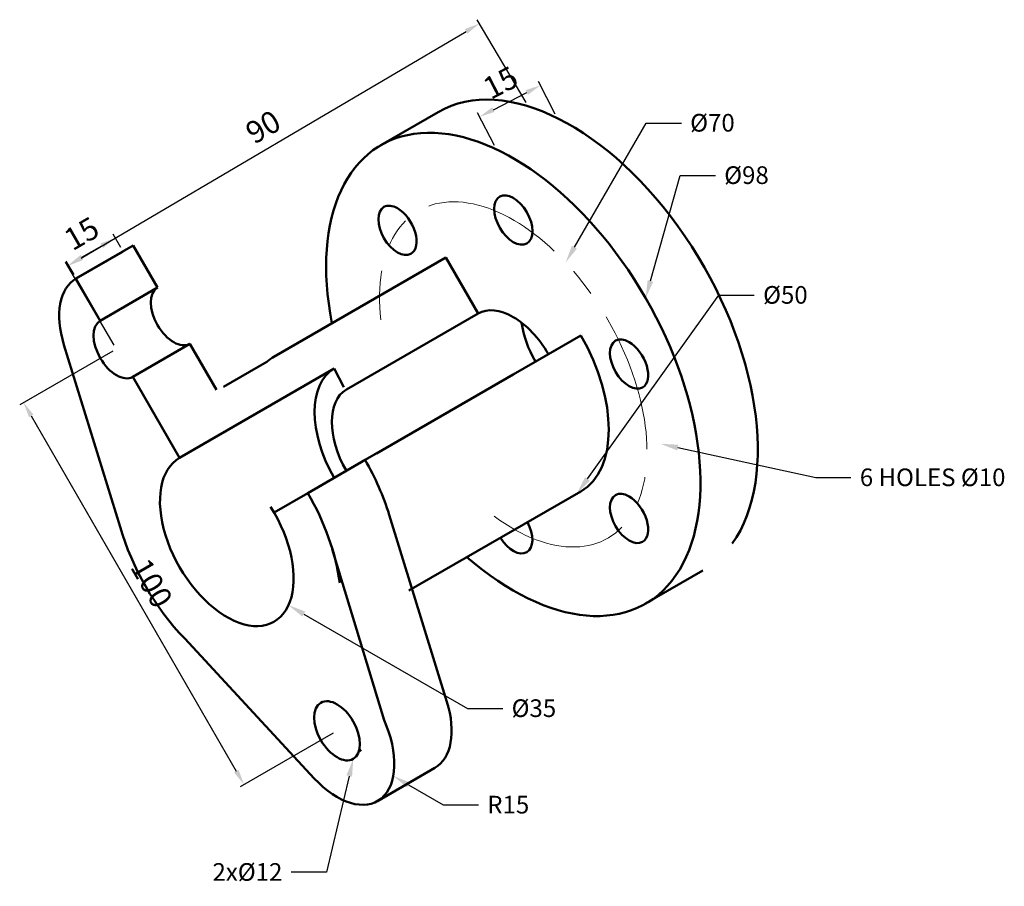
# Model space of a CAD drawing. Units: millimetres. Extents: x 3639 to 3862, y 1643 to 1839.
import ezdxf
from ezdxf import colors
from ezdxf.entities.mleader import LeaderData, LeaderLine
from ezdxf.math import Vec2, Vec3

# ---------------------------------------------------------------- set-up
doc = ezdxf.new("R2010")
doc.units = ezdxf.units.MM
doc.linetypes.add('CENTER', pattern=[50.8, 31.75, -6.35, 6.35, -6.35])
for name, color, linetype, lineweight in [('M-CNTR', 4, 'CENTER', 18), ('M-DIMS', 3, 'Continuous', 25), ('M-OUTL', 7, 'Continuous', 50)]:
    doc.layers.add(name, color=color, linetype=linetype, lineweight=lineweight)
doc.styles.get("Standard").update_dxf_attribs({"font": 'arial.ttf'})
doc.dimstyles.new('AM_ISO$0', dxfattribs={"dimtxt": 5, "dimasz": 3.5, "dimexe": 1, "dimexo": 1, "dimgap": 1.5, "dimtad": 1, "dimdsep": 46, "dimtxsty": 'Standard', "dimcen": 0, "dimclrd": 256, "dimclre": 256, "dimclrt": 2, "dimadec": 0, "dimazin": 2, "dimtp": 0.1, "dimtm": 0.1, "dimtfac": 0.71, "dimtmove": 0, "dimatfit": 3, "dimfxl": 1, "dimlwd": -1, "dimlwe": -1, "dimarcsym": 1})

# ---------------------------------------------------------------- blocks, each defined once
blk = doc.blocks.new('*D3')
at = {"layer": 'Defpoints', "color": 0, "transparency": 16777216}
for p in [(3660.93, 1764.44), (3710.93, 1677.84), (3689.84, 1665.67)]:
    blk.add_point(p, dxfattribs=at)
at = {"layer": 'M-DIMS', "color": 0, "linetype": 'ByBlock', "transparency": 16777216}
for p, q in [((3660.07, 1763.94), (3638.98, 1751.77)), ((3641.59, 1749.24), (3688.09, 1668.7)), ((3710.07, 1677.34), (3688.98, 1665.17))]:
    blk.add_line(p, q, dxfattribs=at)
at = {"layer": 'M-DIMS', "color": 0, "transparency": 16777216}
for points in [[(3642.1, 1749.53), (3641.09, 1748.95), (3639.84, 1752.27)], [(3688.6, 1668.99), (3687.59, 1668.4), (3689.84, 1665.67)]]:
    blk.add_solid(points, dxfattribs=at)
at = {"layer": 'M-DIMS', "color": 0, "transparency": 16777216, "insert": (3668.35, 1710.99), "char_height": 5, "attachment_point": 5, "rotation": 300}
blk.add_mtext('100', dxfattribs=at)
blk = doc.blocks.new('*D4')
at = {"layer": 'Defpoints', "color": 0, "transparency": 16777216}
for p in [(3743.22, 1838.19), (3754.28, 1819.41), (3660.93, 1764.44)]:
    blk.add_point(p, dxfattribs=at)
at = {"layer": 'M-DIMS', "color": 0, "linetype": 'ByBlock', "transparency": 16777216}
for p, q in [((3753.77, 1820.27), (3742.71, 1839.05)), ((3652.89, 1785), (3740.2, 1836.41)), ((3660.42, 1765.3), (3649.37, 1784.08))]:
    blk.add_line(p, q, dxfattribs=at)
at = {"layer": 'M-DIMS', "color": 0, "transparency": 16777216}
for points in [[(3739.91, 1836.92), (3740.5, 1835.91), (3743.22, 1838.19)], [(3652.59, 1785.5), (3653.18, 1784.49), (3649.87, 1783.22)]]:
    blk.add_solid(points, dxfattribs=at)
at = {"layer": 'M-DIMS', "color": 0, "transparency": 16777216, "insert": (3694.49, 1814.2), "char_height": 5, "attachment_point": 5, "rotation": 30.4939}
blk.add_mtext('90', dxfattribs=at)
blk = doc.blocks.new('*D5')
at = {"layer": 'Defpoints', "color": 0, "transparency": 16777216}
for p in [(3660.65, 1789.57), (3662.42, 1786.51), (3651.81, 1780.39)]:
    blk.add_point(p, dxfattribs=at)
at = {"layer": 'M-DIMS', "color": 0, "linetype": 'ByBlock', "transparency": 16777216}
for p, q in [((3661.92, 1787.38), (3660.15, 1790.44)), ((3653.08, 1785.2), (3657.62, 1787.82)), ((3651.31, 1781.26), (3649.55, 1784.31))]:
    blk.add_line(p, q, dxfattribs=at)
at = {"layer": 'M-DIMS', "color": 0, "transparency": 16777216}
for points in [[(3657.33, 1788.33), (3657.91, 1787.32), (3660.65, 1789.57)], [(3652.78, 1785.7), (3653.37, 1784.69), (3650.05, 1783.45)]]:
    blk.add_solid(points, dxfattribs=at)
at = {"layer": 'M-DIMS', "color": 0, "transparency": 16777216, "insert": (3653.32, 1790.02), "char_height": 5, "attachment_point": 5, "rotation": 30}
blk.add_mtext('15', dxfattribs=at)
blk = doc.blocks.new('*D6')
at = {"layer": 'Defpoints', "color": 0, "transparency": 16777216}
for p in [(3757.03, 1824.16), (3760.86, 1816.76), (3747.08, 1809.64)]:
    blk.add_point(p, dxfattribs=at)
at = {"layer": 'M-DIMS', "color": 0, "linetype": 'ByBlock', "transparency": 16777216}
for p, q in [((3760.4, 1817.65), (3756.58, 1825.05)), ((3746.36, 1818.65), (3753.92, 1822.56)), ((3746.62, 1810.53), (3742.79, 1817.94))]:
    blk.add_line(p, q, dxfattribs=at)
at = {"layer": 'M-DIMS', "color": 0, "transparency": 16777216}
for points in [[(3753.66, 1823.08), (3754.19, 1822.04), (3757.03, 1824.16)], [(3746.09, 1819.17), (3746.63, 1818.14), (3743.25, 1817.05)]]:
    blk.add_solid(points, dxfattribs=at)
at = {"layer": 'M-DIMS', "color": 0, "transparency": 16777216, "insert": (3748.28, 1824.21), "char_height": 5, "attachment_point": 5, "rotation": 27.3109}
blk.add_mtext('15', dxfattribs=at)

msp = doc.modelspace()

# ---------------------------------------------------------------- linework, layer by layer
at = {"layer": 'M-CNTR'}
msp.add_ellipse((3750.883, 1758.642), major_axis=(21.433, -37.123), ratio=0.5773503, start_param=5.3548082, end_param=10.353155, dxfattribs=at)
at = {"layer": 'M-OUTL'}
for p, q in [((3733.867, 1818.114), (3720.877, 1810.614)), ((3664.726, 1787.853), (3651.735, 1780.353)), ((3651.746, 1780.353), (3662.417, 1786.514)), ((3662.417, 1786.514), (3651.81, 1780.389)), ((3670.237, 1778.307), (3664.726, 1787.853)), ((3735.574, 1785.158), (3696.603, 1762.658)), ((3742.912, 1772.431), (3735.564, 1785.159)), ((3657.247, 1770.807), (3651.735, 1780.353)), ((3657.247, 1770.807), (3670.237, 1778.307)), ((3713.034, 1755.181), (3742.912, 1772.431)), ((3717.283, 1739.249), (3766.182, 1767.481)), ((3766.182, 1767.481), (3758.834, 1763.238)), ((3661.769, 1724.066), (3649.015, 1765.349)), ((3664.595, 1758.079), (3677.586, 1765.579)), ((3683.602, 1755.159), (3677.586, 1765.579)), ((3694.996, 1761.512), (3685.147, 1755.825)), ((3758.844, 1763.238), (3750.883, 1758.642)), ((3675.215, 1739.703), (3710.286, 1759.951)), ((3710.286, 1759.951), (3712.456, 1755.751)), ((3675.205, 1739.704), (3664.595, 1758.079)), ((3750.883, 1758.642), (3719.873, 1740.738)), ((3717.283, 1739.249), (3731.712, 1747.579)), ((3717.283, 1739.249), (3704.292, 1731.749)), ((3704.292, 1731.749), (3696.638, 1727.329)), ((3766.192, 1732.125), (3727.221, 1709.625)), ((3735.829, 1684.427), (3722.748, 1726.815)), ((3721.593, 1680.255), (3709.854, 1719.031)), ((3780.879, 1706.67), (3793.87, 1714.17)), ((3676.382, 1698.754), (3705.758, 1667.068)), ((3716.017, 1673.674), (3716.429, 1673.229)), ((3733.097, 1669.431), (3720.107, 1661.931))]:
    msp.add_line(p, q, dxfattribs=at)
for centre, major_axis, start_param, end_param in [((3763.873, 1766.142), (30.006, -51.972), 6.54057, 9.424778), ((3750.883, 1758.642), (30.006, -51.972), 5.247811, 10.4601522), ((3724.623, 1791.297), (3.062, -5.303), 2.3561945, 3.1415927), ((3724.623, 1791.297), (3.062, -5.303), 3.1415927, 6.2831853), ((3724.623, 1791.297), (3.062, -5.303), 0, 2.3561945), ((3660.931, 1764.443), (9.186, -15.91), 3.1346147, 4.3365884), ((3673.911, 1771.943), (3.674, -6.364), 3.1415927, 6.2831853), ((3750.873, 1758.642), (7.961, -13.789), 2.3561945, 3.1415927), ((3660.921, 1764.443), (3.674, -6.364), 3.1415927, 6.2831853), ((3750.873, 1758.642), (7.961, -13.789), 1.5707963, 2.3561945), ((3763.863, 1766.142), (7.961, -13.789), 4.0958636, 4.712389), ((3750.873, 1758.642), (15.309, -26.517), 0, 1.5707963), ((3777.123, 1760.987), (3.062, -5.303), 3.1415927, 6.2831853), ((3777.123, 1760.987), (3.062, -5.303), 2.3561945, 3.1415927), ((3777.123, 1760.987), (3.062, -5.303), 0, 2.3561945), ((3711.912, 1736.142), (15.309, -26.517), 3.1415927, 3.2529466), ((3720.995, 1741.392), (10.717, -18.562), 3.1415927, 4.712389), ((3720.995, 1741.392), (7.961, -13.789), 3.1415927, 4.712389), ((3685.931, 1721.142), (10.717, -18.562), 3.1415927, 7.9243433), ((3698.911, 1728.642), (-18.371, 31.82), 4.3361528, 4.712389), ((3685.931, 1721.142), (18.371, -31.82), 0.9529656, 1.5707963), ((3777.123, 1725.987), (3.062, -5.303), 3.1415927, 6.2831853), ((3777.123, 1725.987), (3.062, -5.303), 2.3561945, 3.1415927), ((3777.123, 1725.987), (3.062, -5.303), 0, 2.3561945), ((3685.931, 1721.142), (18.371, -31.82), 4.3033411, 5.1214368), ((3750.873, 1723.642), (3.062, -5.303), 0, 1.5205226), ((3750.873, 1723.642), (3.062, -5.303), 4.7626627, 6.2831853), ((3723.911, 1685.341), (-9.186, 15.91), 3.1415927, 4.3361529), ((3710.931, 1677.84), (9.186, -15.91), 5.0881896, 7.6767006)]:
    msp.add_ellipse(centre, major_axis=major_axis, ratio=0.5773503, start_param=start_param, end_param=end_param, dxfattribs=at)
for centre, major_axis in [((3750.883, 1793.642), (3.062, -5.303)), ((3710.931, 1677.84), (3.674, -6.364))]:
    msp.add_ellipse(centre, major_axis=major_axis, ratio=0.5773503, dxfattribs=at)

# ---------------------------------------------------------------- dimensions: what is measured, and where the dimension line sits
at = {"layer": 'M-DIMS'}
for p1, p2, distance, text, picture, middle in [((3660.931, 1764.443), (3754.275, 1819.413), 21.792, '90', '*D4', (3694.488, 1814.198)), ((3747.077, 1809.642), (3760.859, 1816.758), 8.336, '15', '*D6', (3748.283, 1824.208)), ((3651.81, 1780.389), (3662.417, 1786.513), 3.53, '15', '*D5', (3653.322, 1790.018))]:
    dim = msp.add_aligned_dim(p1=p1, p2=p2, distance=distance, text=text, dimstyle='AM_ISO$0', override={"dimpost": '', "dimclrd": 0, "dimclre": 0, "dimclrt": 0}, dxfattribs=at)
    dim.commit()
    dim.dimension.update_dxf_attribs({"geometry": picture, "text_midpoint": middle})
dim = msp.add_aligned_dim(p1=(3660.931, 1764.443), p2=(3710.931, 1677.84), distance=-24.35, dimstyle='AM_ISO$0', override={"dimpost": '', "dimclrd": 0, "dimclre": 0, "dimclrt": 0}, dxfattribs=at)
dim.commit()
dim.dimension.update_dxf_attribs({"geometry": '*D3', "text_midpoint": (3668.354, 1710.993)})

# ---------------------------------------------------------------- leaders
ml = msp.add_multileader_mtext('Standard', dxfattribs=at)
ml.set_content('{\\C2;%%C70}', color=256)
ml.set_leader_properties()
ml.build(insert=Vec2(0, 0))
ctx = ml.context
ctx.base_point, ctx.plane_origin = Vec3(3788.979, 1815.602), Vec3(3762.738, 1784.009)
notes = []
notes.append((ctx, [(0, (1, 1, 0), (3780.979, 1815.602), (1, 0), 8, [(0, [(3762.738, 1784.009)], 0, [])])]))
ctx.mtext.insert, ctx.mtext.flow_direction = Vec3(3790.979, 1817.683), 5
ml = msp.add_multileader_mtext('Standard', dxfattribs=at)
ml.set_content('{\\C2;%%C98}', color=256)
ml.set_leader_properties()
ml.build(insert=Vec2(0, 0))
ctx = ml.context
ctx.base_point, ctx.plane_origin = Vec3(3796.7, 1803.733), Vec3(3780.889, 1775.966)
notes.append((ctx, [(0, (1, 1, 0), (3788.7, 1803.733), (1, 0), 8, [(0, [(3780.889, 1775.966)], 0, [])])]))
ctx.mtext.insert, ctx.mtext.flow_direction = Vec3(3798.7, 1805.814), 5
ml = msp.add_multileader_mtext('Standard', dxfattribs=at)
ml.set_content('{\\C2;%%C50}', color=256)
ml.set_leader_properties()
ml.build(insert=Vec2(0, 0))
ctx = ml.context
ctx.base_point, ctx.plane_origin = Vec3(3805.514, 1776.587), Vec3(3771.111, 1755.874)
notes.append((ctx, [(0, (1, 1, 0), (3797.514, 1776.587), (1, 0), 8, [(0, [(3765.351, 1731.69)], 0, [])])]))
ctx.mtext.insert, ctx.mtext.flow_direction = Vec3(3807.514, 1778.667), 5
ml = msp.add_multileader_mtext('Standard', dxfattribs=at)
ml.set_content('{\\C2;6 HOLES %%C10}', color=256)
ml.set_leader_properties()
ml.build(insert=Vec2(0, 0))
ctx = ml.context
ctx.base_point, ctx.plane_origin = Vec3(3827.434, 1735.233), Vec3(3784.256, 1742.909)
notes.append((ctx, [(0, (1, 1, 0), (3819.434, 1735.233), (1, 0), 8, [(0, [(3784.256, 1742.909)], 0, [])])]))
ctx.mtext.insert, ctx.mtext.flow_direction = Vec3(3829.434, 1737.313), 5
ml = msp.add_multileader_mtext('Standard', dxfattribs=at)
ml.set_content('{\\C2;%%C35}', color=256)
ml.set_leader_properties()
ml.build(insert=Vec2(0, 0))
ctx = ml.context
ctx.base_point, ctx.plane_origin = Vec3(3748.5, 1682.893), Vec3(3699.916, 1706.324)
notes.append((ctx, [(0, (1, 1, 0), (3740.5, 1682.893), (1, 0), 8, [(0, [(3699.916, 1706.324)], 0, [])])]))
ctx.mtext.insert, ctx.mtext.flow_direction = Vec3(3750.5, 1684.973), 5
ml = msp.add_multileader_mtext('Standard', dxfattribs=at)
ml.set_content('{\\C2;2x%%C12}', color=256)
ml.set_leader_properties()
ml.build(insert=Vec2(0, 0))
ctx = ml.context
ctx.base_point, ctx.plane_origin = Vec3(3680.528, 1645.764), Vec3(3714.605, 1671.476)
ctx.text_align_type = 2
notes.append((ctx, [(0, (1, 1, 0), (3708.533, 1645.764), (-1, 0), 8, [(0, [(3714.605, 1671.476)], 0, [])])]))
ctx.mtext.insert, ctx.mtext.alignment, ctx.mtext.flow_direction = Vec3(3698.533, 1647.844), 3, 5
ml = msp.add_multileader_mtext('Standard', dxfattribs=at)
ml.set_content('{\\C2;R15}', color=256)
ml.set_leader_properties()
ml.build(insert=Vec2(0, 0))
ctx = ml.context
ctx.base_point, ctx.plane_origin = Vec3(3742.974, 1661.07), Vec3(3723.678, 1667.592)
notes.append((ctx, [(0, (1, 1, 0), (3734.974, 1661.07), (1, 0), 8, [(0, [(3723.678, 1667.592)], 0, [])])]))
ctx.mtext.insert, ctx.mtext.flow_direction = Vec3(3744.974, 1663.105), 5
for ctx, leaders in notes:
    for number, flags, end, landing, length, lines in leaders:
        leader = LeaderData()
        leader.index, (leader.has_last_leader_line, leader.has_dogleg_vector, leader.attachment_direction) = number, flags
        leader.last_leader_point, leader.dogleg_vector, leader.dogleg_length = Vec3(end), Vec3(landing), length
        for number, points, colour, breaks in lines:
            line = LeaderLine()
            line.index, line.vertices, line.color, line.breaks = number, Vec3.list(points), colors.encode_raw_color(colour), breaks
            leader.lines.append(line)
        ctx.leaders.append(leader)

doc.saveas('drawing.dxf')
